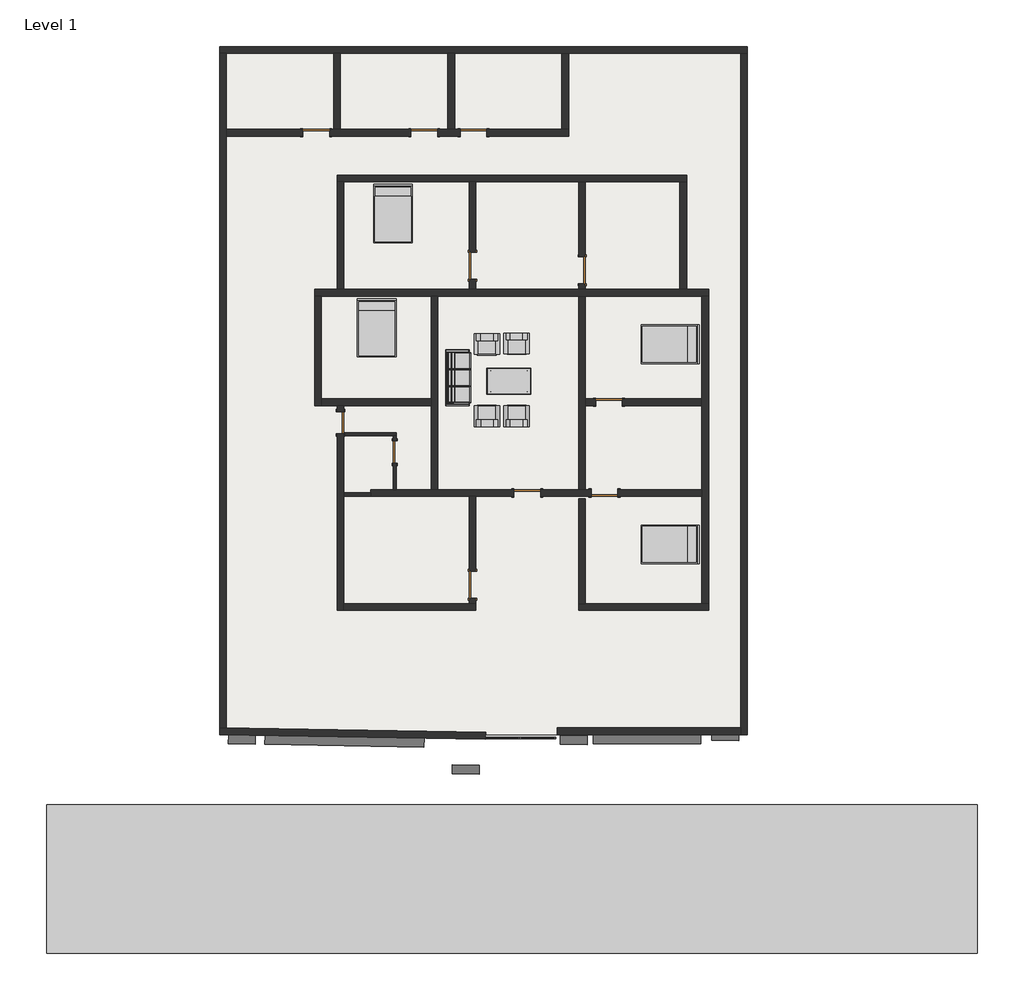
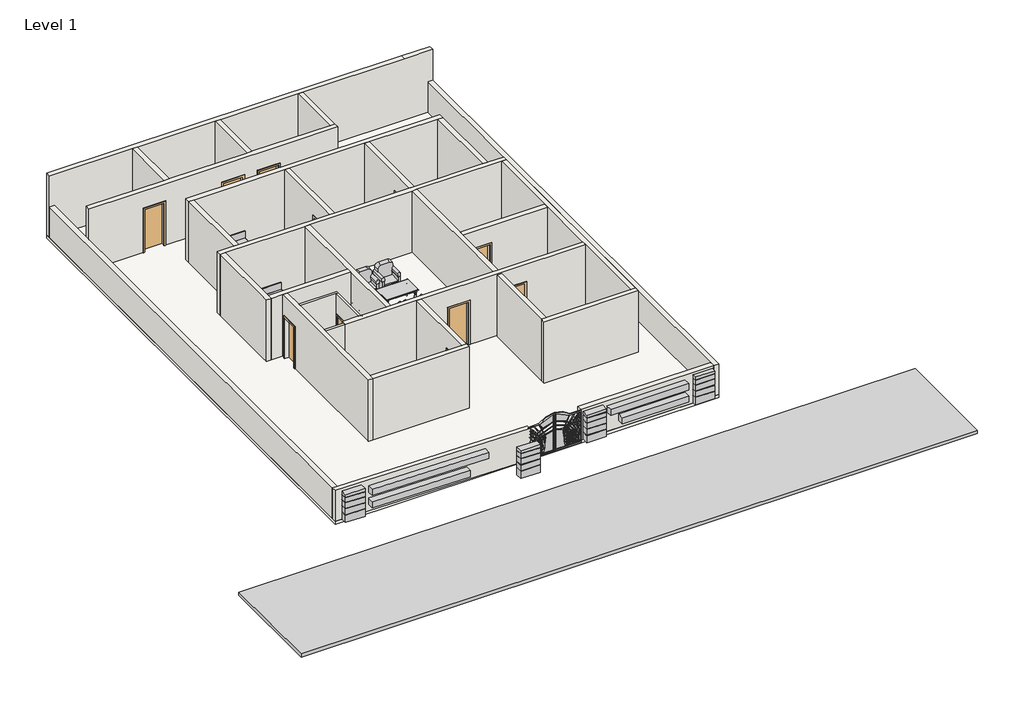
# One storey, incomplete: 30 walls, 11 doors, 10 furniture elements, 8 proxies, 1 slab.
"""IFC4 building model written with IfcOpenShell, lengths in millimetres."""

from ifc_helpers import new_model, si_unit, frame, origin, origin_with_axes, place, context, project, spatial, polyline, outline, extrude, faceted_brep, transform, mapped, element, save
from components import generic_models_6bc30956, generic_models_1_generic_models_1_9302cbdc, generic_models_2_generic_models_2_68b0420d, generic_models_3_generic_models_1_5bebd585, generic_models_4_generic_models_1_1a32cfe3, generic_models_5_generic_models_1_3fb950e5, generic_models_6_generic_models_6_20551735, generic_models_7_generic_models_7_4119f6ec, door_a1484949, door_d8f5dbb5, door_0ca8825f, door_a90ba1ad, furniture_2fc85b74, furniture_29a9adb8, furniture_57072a26, bed_17739_bed_17739_15c61121, chair_lounge_11461_couch_0866092f, dining_table_14755_dining_table_14755_d89cb775

model = new_model("IFC4")

# Units and contexts
model_context = context("Model", 3, world=origin())
ifc_project = project(units=[si_unit("LENGTHUNIT", "METRE", prefix="MILLI")], contexts=[model_context])

# Site, building, storey
site = spatial("IfcSite", under=ifc_project)
building = spatial("IfcBuilding", under=site)
storey = spatial("IfcBuildingStorey", under=building, Name="Level 1", Elevation=0.0)

# Proxies
placement = place(None, origin())
generic_models_shape = generic_models_6bc30956(model_context)
element("IfcBuildingElementProxy", 1, Name="Generic Models", at=placement, inside=storey, context=model_context, shape_type="MappedRepresentation", body=[
    mapped(generic_models_shape, transform((-28.292132, -11258.8237368, 0.0), x_axis=(1.0, 0.0, 0.0), y_axis=(0.0, 1.0, 0.0), z_axis=(0.0, 0.0, 1.0))),
])
generic_models_1_generic_models_1_shape = generic_models_1_generic_models_1_9302cbdc(model_context)
element("IfcBuildingElementProxy", 2, Name="Generic Models 1 : Generic Models 1", ObjectType="Generic Models 1 : Generic Models 1", at=placement, inside=storey, context=model_context, shape_type="MappedRepresentation", body=[
    mapped(generic_models_1_generic_models_1_shape, transform((0.0, 0.0, 0.0), x_axis=(1.0, 0.0, 0.0), y_axis=(0.0, 1.0, 0.0), z_axis=(0.0, 0.0, 1.0))),
])
generic_models_2_generic_models_2_shape = generic_models_2_generic_models_2_68b0420d(model_context)
element("IfcBuildingElementProxy", 3, Name="Generic Models 2 : Generic Models 2", ObjectType="Generic Models 2 : Generic Models 2", at=placement, inside=storey, context=model_context, shape_type="MappedRepresentation", body=[
    mapped(generic_models_2_generic_models_2_shape, transform((0.0, 0.0, 0.0), x_axis=(1.0, 0.0, 0.0), y_axis=(0.0, 1.0, 0.0), z_axis=(0.0, 0.0, 1.0))),
])
generic_models_3_generic_models_1_shape = generic_models_3_generic_models_1_5bebd585(model_context)
element("IfcBuildingElementProxy", 4, Name="Generic Models 3 : Generic Models 1", ObjectType="Generic Models 3 : Generic Models 1", at=placement, inside=storey, context=model_context, shape_type="MappedRepresentation", body=[
    mapped(generic_models_3_generic_models_1_shape, transform((0.0, 0.0, 0.0), x_axis=(1.0, 0.0, 0.0), y_axis=(0.0, 1.0, 0.0), z_axis=(0.0, 0.0, 1.0))),
])
generic_models_4_generic_models_1_shape = generic_models_4_generic_models_1_1a32cfe3(model_context)
element("IfcBuildingElementProxy", 5, Name="Generic Models 4 : Generic Models 1", ObjectType="Generic Models 4 : Generic Models 1", at=placement, inside=storey, context=model_context, shape_type="MappedRepresentation", body=[
    mapped(generic_models_4_generic_models_1_shape, transform((0.0, 0.0, 0.0), x_axis=(1.0, 0.0, 0.0), y_axis=(0.0, 1.0, 0.0), z_axis=(0.0, 0.0, 1.0))),
])
generic_models_5_generic_models_1_shape = generic_models_5_generic_models_1_3fb950e5(model_context)
element("IfcBuildingElementProxy", 6, Name="Generic Models 5 : Generic Models 1", ObjectType="Generic Models 5 : Generic Models 1", at=placement, inside=storey, context=model_context, shape_type="MappedRepresentation", body=[
    mapped(generic_models_5_generic_models_1_shape, transform((0.0, 0.0, 0.0), x_axis=(1.0, 0.0, 0.0), y_axis=(0.0, 1.0, 0.0), z_axis=(0.0, 0.0, 1.0))),
])
generic_models_6_generic_models_6_shape = generic_models_6_generic_models_6_20551735(model_context)
element("IfcBuildingElementProxy", 7, Name="Generic Models 6 : Generic Models 6", ObjectType="Generic Models 6 : Generic Models 6", at=placement, inside=storey, context=model_context, shape_type="MappedRepresentation", body=[
    mapped(generic_models_6_generic_models_6_shape, transform((0.0, 0.0, 0.0), x_axis=(1.0, 0.0, 0.0), y_axis=(0.0, 1.0, 0.0), z_axis=(0.0, 0.0, 1.0))),
])
generic_models_7_generic_models_7_shape = generic_models_7_generic_models_7_4119f6ec(model_context)
element("IfcBuildingElementProxy", 8, Name="Generic Models 7 : Generic Models 7", ObjectType="Generic Models 7 : Generic Models 7", at=placement, inside=storey, context=model_context, shape_type="MappedRepresentation", body=[
    mapped(generic_models_7_generic_models_7_shape, transform((0.0, 0.0, 0.0), x_axis=(1.0, 0.0, 0.0), y_axis=(0.0, 1.0, 0.0), z_axis=(0.0, 0.0, 1.0))),
])

# Doors
door_shape = door_a1484949(model_context)
element("IfcDoor", 9, ObjectType="Single-Flush : 30\" x 80\"", at=placement, inside=storey, context=model_context, shape_type="MappedRepresentation", body=[
    mapped(door_shape, transform((-6124.8057305, -546.3292186, 0.0), x_axis=(0.0, -1.0, 0.0), y_axis=(1.0, 0.0, 0.0), z_axis=(0.0, 0.0, 1.0))),
])
door_2_shape = door_d8f5dbb5(model_context)
element("IfcDoor", 10, ObjectType="Single-Flush : 30\" x 80\"", at=placement, inside=storey, context=model_context, shape_type="MappedRepresentation", body=[
    mapped(door_2_shape, transform((-4276.442132, -1546.4542186, 0.0), x_axis=(0.0, 1.0, 0.0), y_axis=(-1.0, 0.0, 0.0), z_axis=(0.0, 0.0, 1.0))),
])
door_3_shape = door_0ca8825f(model_context)
element("IfcDoor", 11, ObjectType="Single-Flush : 36\" x 84\"", at=placement, inside=storey, context=model_context, shape_type="MappedRepresentation", body=[
    mapped(door_3_shape, transform((-6952.8959326, 9329.2722985, 0.0), x_axis=(1.0, 0.0, 0.0), y_axis=(0.0, 1.0, 0.0), z_axis=(0.0, 0.0, 1.0))),
])
element("IfcDoor", 12, ObjectType="Single-Flush : 36\" x 84\"", at=placement, inside=storey, context=model_context, shape_type="MappedRepresentation", body=[
    mapped(door_3_shape, transform((-3267.5476203, 9329.2722985, 0.0), x_axis=(1.0, 0.0, 0.0), y_axis=(0.0, 1.0, 0.0), z_axis=(0.0, 0.0, 1.0))),
])
element("IfcDoor", 13, ObjectType="Single-Flush : 36\" x 84\"", at=placement, inside=storey, context=model_context, shape_type="MappedRepresentation", body=[
    mapped(door_3_shape, transform((2105.307868, 4644.7957814, 0.0), x_axis=(0.0, -1.0, 0.0), y_axis=(1.0, 0.0, 0.0), z_axis=(0.0, 0.0, 1.0))),
])
element("IfcDoor", 14, ObjectType="Single-Flush : 36\" x 84\"", at=placement, inside=storey, context=model_context, shape_type="MappedRepresentation", body=[
    mapped(door_3_shape, transform((2867.307868, -2937.1042186, 0.0), x_axis=(-1.0, 0.0, 0.0), y_axis=(0.0, -1.0, 0.0), z_axis=(0.0, 0.0, 1.0))),
])
element("IfcDoor", 15, ObjectType="Single-Flush : 36\" x 84\"", at=placement, inside=storey, context=model_context, shape_type="MappedRepresentation", body=[
    mapped(door_3_shape, transform((238.407868, -2937.1042186, 0.0), x_axis=(1.0, 0.0, 0.0), y_axis=(0.0, 1.0, 0.0), z_axis=(0.0, 0.0, 1.0))),
])
door_4_shape = door_a90ba1ad(model_context)
element("IfcDoor", 16, ObjectType="Single-Flush : 36\" x 84\"", at=placement, inside=storey, context=model_context, shape_type="MappedRepresentation", body=[
    mapped(door_4_shape, transform((-1591.1476203, 9329.2722985, 0.0), x_axis=(-1.0, 0.0, 0.0), y_axis=(0.0, -1.0, 0.0), z_axis=(0.0, 0.0, 1.0))),
])
element("IfcDoor", 17, ObjectType="Single-Flush : 36\" x 84\"", at=placement, inside=storey, context=model_context, shape_type="MappedRepresentation", body=[
    mapped(door_4_shape, transform((-1628.492132, 4797.1957814, 0.0), x_axis=(0.0, -1.0, 0.0), y_axis=(1.0, 0.0, 0.0), z_axis=(0.0, 0.0, 1.0))),
])
element("IfcDoor", 18, ObjectType="Single-Flush : 36\" x 84\"", at=placement, inside=storey, context=model_context, shape_type="MappedRepresentation", body=[
    mapped(door_4_shape, transform((3019.707868, 148.9957814, 0.0), x_axis=(-1.0, 0.0, 0.0), y_axis=(0.0, -1.0, 0.0), z_axis=(0.0, 0.0, 1.0))),
])
element("IfcDoor", 19, ObjectType="Single-Flush : 36\" x 84\"", at=placement, inside=storey, context=model_context, shape_type="MappedRepresentation", body=[
    mapped(door_4_shape, transform((-1628.492132, -6061.3042186, 0.0), x_axis=(0.0, -1.0, 0.0), y_axis=(1.0, 0.0, 0.0), z_axis=(0.0, 0.0, 1.0))),
])

# Furniture
furniture_shape = furniture_2fc85b74(model_context)
furniture_2_shape = furniture_29a9adb8(model_context)
furniture_3_shape = furniture_57072a26(model_context)
element("IfcFurniture", 20, at=placement, inside=storey, context=model_context, shape_type="MappedRepresentation", body=[
    mapped(furniture_shape, transform((-1742.792132, 987.1957814, 0.0), x_axis=(0.0, 1.0, 0.0), y_axis=(-1.0, 0.0, 0.0), z_axis=(0.0, 0.0, 1.0))),
    mapped(furniture_2_shape, transform((-1742.792132, 987.1957814, 0.0), x_axis=(0.0, 1.0, 0.0), y_axis=(-1.0, 0.0, 0.0), z_axis=(0.0, 0.0, 1.0))),
    mapped(furniture_3_shape, transform((-1742.792132, 987.1957814, 0.0), x_axis=(0.0, 1.0, 0.0), y_axis=(-1.0, 0.0, 0.0), z_axis=(0.0, 0.0, 1.0))),
])
bed_17739_bed_17739_shape = bed_17739_bed_17739_15c61121(model_context)
element("IfcFurniture", 21, ObjectType="Bed_17739 : Bed_17739", at=placement, inside=storey, context=model_context, shape_type="MappedRepresentation", body=[
    mapped(bed_17739_bed_17739_shape, transform((-4333.592132, 6549.7957814, 0.0), x_axis=(1.0, 0.0, 0.0), y_axis=(0.0, 1.0, 0.0), z_axis=(0.0, 0.0, 1.0))),
])
element("IfcFurniture", 22, ObjectType="Bed_17739 : Bed_17739", at=placement, inside=storey, context=model_context, shape_type="MappedRepresentation", body=[
    mapped(bed_17739_bed_17739_shape, transform((5077.107868, 2130.1957814, 0.0), x_axis=(0.0, -1.0, 0.0), y_axis=(1.0, 0.0, 0.0), z_axis=(0.0, 0.0, 1.0))),
])
element("IfcFurniture", 23, ObjectType="Bed_17739 : Bed_17739", at=placement, inside=storey, context=model_context, shape_type="MappedRepresentation", body=[
    mapped(bed_17739_bed_17739_shape, transform((5077.107868, -4689.7042186, 0.0), x_axis=(0.0, -1.0, 0.0), y_axis=(1.0, 0.0, 0.0), z_axis=(0.0, 0.0, 1.0))),
])
element("IfcFurniture", 24, ObjectType="Bed_17739 : Bed_17739", at=placement, inside=storey, context=model_context, shape_type="MappedRepresentation", body=[
    mapped(bed_17739_bed_17739_shape, transform((-4886.042132, 2663.5957814, 0.0), x_axis=(1.0, 0.0, 0.0), y_axis=(0.0, 1.0, 0.0), z_axis=(0.0, 0.0, 1.0))),
])
chair_lounge_11461_couch_shape = chair_lounge_11461_couch_0866092f(model_context)
element("IfcFurniture", 25, ObjectType="Chair-Lounge_11461 : Couch", at=placement, inside=storey, context=model_context, shape_type="MappedRepresentation", body=[
    mapped(chair_lounge_11461_couch_shape, transform((-1135.6501746, 2478.1239494, 0.0), x_axis=(1.0, 0.0, 0.0), y_axis=(0.0, 1.0, 0.0), z_axis=(0.0, 0.0, 1.0))),
])
element("IfcFurniture", 26, ObjectType="Chair-Lounge_11461 : Couch", at=placement, inside=storey, context=model_context, shape_type="MappedRepresentation", body=[
    mapped(chair_lounge_11461_couch_shape, transform((-1135.6501746, -676.3685812, 0.0), x_axis=(-1.0, 0.0, 0.0), y_axis=(0.0, -1.0, 0.0), z_axis=(0.0, 0.0, 1.0))),
])
element("IfcFurniture", 27, ObjectType="Chair-Lounge_11461 : Couch", at=placement, inside=storey, context=model_context, shape_type="MappedRepresentation", body=[
    mapped(chair_lounge_11461_couch_shape, transform((-125.9107827, -676.3685812, 0.0), x_axis=(-1.0, 0.0, 0.0), y_axis=(0.0, -1.0, 0.0), z_axis=(0.0, 0.0, 1.0))),
])
element("IfcFurniture", 28, ObjectType="Chair-Lounge_11461 : Couch", at=placement, inside=storey, context=model_context, shape_type="MappedRepresentation", body=[
    mapped(chair_lounge_11461_couch_shape, transform((-125.9107827, 2504.7969663, 0.0), x_axis=(1.0, 0.0, 0.0), y_axis=(0.0, 1.0, 0.0), z_axis=(0.0, 0.0, 1.0))),
])
dining_table_14755_dining_table_14755_shape = dining_table_14755_dining_table_14755_d89cb775(model_context)
element("IfcFurniture", 29, ObjectType="Dining_table_14755 : Dining_table_14755", at=placement, inside=storey, context=model_context, shape_type="MappedRepresentation", body=[
    mapped(dining_table_14755_dining_table_14755_shape, transform((-1135.6501746, 415.6957814, 0.0), x_axis=(1.0, 0.0, 0.0), y_axis=(0.0, 1.0, 0.0), z_axis=(0.0, 0.0, 1.0))),
])

# Slab
element("IfcSlab", 30, ObjectType="Generic - 12\"", at=placement, inside=storey, context=model_context, shape_type="SweptSolid", body=[
    extrude(outline(polyline([(7729.3646036, 12262.9722985), (7729.3646036, -11166.6749898), (-10239.8476203, -11166.6749898), (-10239.8476203, 12262.9722985), (7729.3646036, 12262.9722985)])), frame((0.0, 0.0, -152.4), z_axis=(0.0, 0.0, 1.0), x_axis=(1.0, 0.0, 0.0)), (0.0, 0.0, 1.0), 152.4),
])

# Walls
element("IfcWall", 31, ObjectType="4.5\"WALL", at=placement, inside=storey, context=model_context, shape_type="Brep", body=[
    faceted_brep([(-6010.5057305, -994.0042186, 0.0), (-4333.592132, -994.0042186, 0.0), (-4219.292132, -994.0042186, 0.0), (-4219.292132, -994.0042186, 3048.0), (-4333.592132, -994.0042186, 3048.0), (-6010.5057305, -994.0042186, 3048.0), (-6010.5057305, -879.7042186, 0.0), (-6010.5057305, -879.7042186, 3048.0), (-4219.292132, -879.7042186, 3048.0), (-4219.292132, -879.7042186, 0.0)], [[[0, 1, 2, 3, 4, 5]], [[6, 7, 8, 9]], [[2, 1, 0, 6, 9]], [[0, 5, 7, 6]], [[3, 2, 9, 8]], [[5, 4, 3, 8, 7]]]),
])
element("IfcWall", 32, ObjectType="4.5\"WALL", at=placement, inside=storey, context=model_context, shape_type="SweptSolid", body=[
    extrude(outline(polyline([(-994.0042186, 0.0), (-1165.4542186, 0.0), (-1165.4542186, 2032.0), (-1927.4542186, 2032.0), (-1927.4542186, 0.0), (-2822.8042186, 0.0), (-2822.8042186, 3048.0), (-994.0042186, 3048.0), (-994.0042186, 0.0)])), frame((-4333.592132, 0.0, 0.0), z_axis=(1.0, 0.0, 0.0), x_axis=(0.0, 1.0, 0.0)), (0.0, 0.0, 1.0), 114.3),
])
element("IfcWall", 33, ObjectType="4.5\"WALL", at=placement, inside=storey, context=model_context, shape_type="SweptSolid", body=[
    extrude(outline(polyline([(-5096.0236102, -3051.4042186), (-6010.5057305, -3051.4042186), (-6010.5057305, -2937.1042186), (-5096.0236102, -2937.1042186), (-5096.0236102, -3051.4042186)])), origin_with_axes(), (0.0, 0.0, 1.0), 3048.0),
])
element("IfcWall", 34, ObjectType="WALL9\"", at=placement, inside=storey, context=model_context, shape_type="Brep", body=[
    faceted_brep([(-10239.8476203, 12034.3722985, 0.0), (-10011.2476203, 12034.3722985, 0.0), (-6353.6476203, 12034.3722985, 0.0), (-6125.0476203, 12034.3722985, 0.0), (-2467.4476203, 12034.3722985, 0.0), (-2238.8476203, 12034.3722985, 0.0), (1418.7523797, 12034.3722985, 0.0), (1647.3523797, 12034.3722985, 0.0), (7500.7646036, 12034.3722985, 0.0), (7729.3646036, 12034.3722985, 0.0), (7729.3646036, 12034.3722985, 1524.0), (7729.3646036, 12034.3722985, 3048.0), (6410.607868, 12034.3722985, 3048.0), (1647.3523797, 12034.3722985, 3048.0), (1418.7523797, 12034.3722985, 3048.0), (-2238.8476203, 12034.3722985, 3048.0), (-2467.4476203, 12034.3722985, 3048.0), (-6125.0476203, 12034.3722985, 3048.0), (-6353.6476203, 12034.3722985, 3048.0), (-10239.8476203, 12034.3722985, 3048.0), (-10239.8476203, 12034.3722985, 1524.0), (-10239.8476203, 12262.9722985, 0.0), (-10239.8476203, 12262.9722985, 3048.0), (6410.607868, 12262.9722985, 3048.0), (7729.3646036, 12262.9722985, 3048.0), (7729.3646036, 12262.9722985, 0.0)], [[[0, 1, 2, 3, 4, 5, 6, 7, 8, 9, 10, 11, 12, 13, 14, 15, 16, 17, 18, 19, 20]], [[21, 22, 23, 24, 25]], [[9, 8, 7, 6, 5, 4, 3, 2, 1, 0, 21, 25]], [[11, 10, 9, 25, 24]], [[12, 11, 24, 23]], [[19, 18, 17, 16, 15, 14, 13, 12, 23, 22]], [[0, 20, 19, 22, 21]]]),
])
element("IfcWall", 35, ObjectType="WALL9\"", at=placement, inside=storey, context=model_context, shape_type="Brep", body=[
    faceted_brep([(7500.7646036, 12034.3722985, 0.0), (7500.7646036, -10938.0749898, 0.0), (7500.7646036, -11166.6749898, 0.0), (7500.7646036, -11166.6749898, 1524.0), (7500.7646036, -10938.0749898, 1524.0), (7500.7646036, 12034.3722985, 1524.0), (7729.3646036, 12034.3722985, 0.0), (7729.3646036, 12034.3722985, 1524.0), (7729.3646036, -11166.6749898, 1524.0), (7729.3646036, -11166.6749898, 0.0)], [[[0, 1, 2, 3, 4, 5]], [[6, 7, 8, 9]], [[2, 1, 0, 6, 9]], [[5, 4, 3, 8, 7]], [[0, 5, 7, 6]], [[3, 2, 9, 8]]]),
])
element("IfcWall", 36, ObjectType="WALL9\"", at=placement, inside=storey, context=model_context, shape_type="SweptSolid", body=[
    extrude(outline(polyline([(1265.0646036, -10938.0749898), (7500.7646036, -10938.0749898), (7500.7646036, -11166.6749898), (1265.0646036, -11166.6749898), (1265.0646036, -10938.0749898)])), origin_with_axes(), (0.0, 0.0, 1.0), 1524.0),
])
element("IfcWall", 37, ObjectType="WALL9\"", at=placement, inside=storey, context=model_context, shape_type="Brep", body=[
    faceted_brep([(-2810.3476203, 9214.9722985, 0.0), (-2048.3476203, 9214.9722985, 0.0), (-2048.3476203, 9214.9722985, 2133.6), (-1133.9476203, 9214.9722985, 2133.6), (-1133.9476203, 9214.9722985, 0.0), (1647.3523797, 9214.9722985, 0.0), (1647.3523797, 9214.9722985, 3048.0), (-6238.592132, 9214.9722985, 3048.0), (-10011.2476203, 9214.9722985, 3048.0), (-10011.2476203, 9214.9722985, 0.0), (-7410.0959326, 9214.9722985, 0.0), (-7410.0959326, 9214.9722985, 2133.6), (-6495.6959326, 9214.9722985, 2133.6), (-6495.6959326, 9214.9722985, 0.0), (-3724.7476203, 9214.9722985, 0.0), (-3724.7476203, 9214.9722985, 2133.6), (-2810.3476203, 9214.9722985, 2133.6), (-2048.3476203, 9443.5722985, 2133.6), (-2048.3476203, 9443.5722985, 0.0), (-2238.8476203, 9443.5722985, 0.0), (-2467.4476203, 9443.5722985, 0.0), (-2810.3476203, 9443.5722985, 0.0), (-2810.3476203, 9443.5722985, 2133.6), (-3724.7476203, 9443.5722985, 2133.6), (-3724.7476203, 9443.5722985, 0.0), (-6125.0476203, 9443.5722985, 0.0), (-6353.6476203, 9443.5722985, 0.0), (-6495.6959326, 9443.5722985, 0.0), (-6495.6959326, 9443.5722985, 2133.6), (-7410.0959326, 9443.5722985, 2133.6), (-7410.0959326, 9443.5722985, 0.0), (-10011.2476203, 9443.5722985, 0.0), (-10011.2476203, 9443.5722985, 3048.0), (-6353.6476203, 9443.5722985, 3048.0), (-6125.0476203, 9443.5722985, 3048.0), (-2467.4476203, 9443.5722985, 3048.0), (-2238.8476203, 9443.5722985, 3048.0), (1418.7523797, 9443.5722985, 3048.0), (1647.3523797, 9443.5722985, 3048.0), (1647.3523797, 9443.5722985, 0.0), (1418.7523797, 9443.5722985, 0.0), (-1133.9476203, 9443.5722985, 0.0), (-1133.9476203, 9443.5722985, 2133.6)], [[[0, 1, 2, 3, 4, 5, 6, 7, 8, 9, 10, 11, 12, 13, 14, 15, 16]], [[17, 18, 19, 20, 21, 22, 23, 24, 25, 26, 27, 28, 29, 30, 31, 32, 33, 34, 35, 36, 37, 38, 39, 40, 41, 42]], [[10, 9, 31, 30]], [[14, 13, 27, 26, 25, 24]], [[41, 40, 39, 5, 4]], [[21, 20, 19, 18, 1, 0]], [[6, 5, 39, 38]], [[28, 27, 13, 12]], [[29, 28, 12, 11]], [[30, 29, 11, 10]], [[22, 21, 0, 16]], [[23, 22, 16, 15]], [[24, 23, 15, 14]], [[2, 1, 18, 17]], [[3, 2, 17, 42]], [[4, 3, 42, 41]], [[8, 7, 6, 38, 37, 36, 35, 34, 33, 32]], [[9, 8, 32, 31]]]),
])
element("IfcWall", 38, ObjectType="WALL9\"", at=placement, inside=storey, context=model_context, shape_type="SweptSolid", body=[
    extrude(outline(polyline([(1647.3523797, 12034.3722985), (1647.3523797, 9443.5722985), (1418.7523797, 9443.5722985), (1418.7523797, 12034.3722985), (1647.3523797, 12034.3722985)])), origin_with_axes(), (0.0, 0.0, 1.0), 3048.0),
])
element("IfcWall", 39, ObjectType="WALL9\"", at=placement, inside=storey, context=model_context, shape_type="SweptSolid", body=[
    extrude(outline(polyline([(-2467.4476203, 9443.5722985), (-2467.4476203, 12034.3722985), (-2238.8476203, 12034.3722985), (-2238.8476203, 9443.5722985), (-2467.4476203, 9443.5722985)])), origin_with_axes(), (0.0, 0.0, 1.0), 3048.0),
])
element("IfcWall", 40, ObjectType="WALL9\"", at=placement, inside=storey, context=model_context, shape_type="SweptSolid", body=[
    extrude(outline(polyline([(-6353.6476203, 9443.5722985), (-6353.6476203, 12034.3722985), (-6125.0476203, 12034.3722985), (-6125.0476203, 9443.5722985), (-6353.6476203, 9443.5722985)])), origin_with_axes(), (0.0, 0.0, 1.0), 3048.0),
])
element("IfcWall", 41, ObjectType="WALL9\"", at=placement, inside=storey, context=model_context, shape_type="Brep", body=[
    faceted_brep([(-6238.592132, 7654.6957814, 0.0), (-6009.992132, 7654.6957814, 0.0), (-1742.792132, 7654.6957814, 0.0), (-1514.192132, 7654.6957814, 0.0), (1991.007868, 7654.6957814, 0.0), (2219.607868, 7654.6957814, 0.0), (5432.707868, 7654.6957814, 0.0), (5661.307868, 7654.6957814, 0.0), (5661.307868, 7654.6957814, 3048.0), (5432.707868, 7654.6957814, 3048.0), (2219.607868, 7654.6957814, 3048.0), (1991.007868, 7654.6957814, 3048.0), (-1514.192132, 7654.6957814, 3048.0), (-1742.792132, 7654.6957814, 3048.0), (-6009.992132, 7654.6957814, 3048.0), (-6238.592132, 7654.6957814, 3048.0), (-6238.592132, 7883.2957814, 0.0), (-6238.592132, 7883.2957814, 3048.0), (5661.307868, 7883.2957814, 3048.0), (5661.307868, 7883.2957814, 0.0)], [[[0, 1, 2, 3, 4, 5, 6, 7, 8, 9, 10, 11, 12, 13, 14, 15]], [[16, 17, 18, 19]], [[7, 6, 5, 4, 3, 2, 1, 0, 16, 19]], [[0, 15, 17, 16]], [[15, 14, 13, 12, 11, 10, 9, 8, 18, 17]], [[8, 7, 19, 18]]]),
])
element("IfcWall", 42, ObjectType="WALL9\"", at=placement, inside=storey, context=model_context, shape_type="SweptSolid", body=[
    extrude(outline(polyline([(-6238.592132, 3997.0957814), (-6238.592132, 7654.6957814), (-6009.992132, 7654.6957814), (-6009.992132, 3997.0957814), (-6238.592132, 3997.0957814)])), origin_with_axes(), (0.0, 0.0, 1.0), 3048.0),
])
element("IfcWall", 43, ObjectType="WALL9\"", at=placement, inside=storey, context=model_context, shape_type="SweptSolid", body=[
    extrude(outline(polyline([(4339.9957814, 2133.6), (4339.9957814, 0.0), (3997.0957814, 0.0), (3997.0957814, 3048.0), (7654.6957814, 3048.0), (7654.6957814, 0.0), (5254.3957814, 0.0), (5254.3957814, 2133.6), (4339.9957814, 2133.6)])), frame((-1742.792132, 0.0, 0.0), z_axis=(1.0, 0.0, 0.0), x_axis=(0.0, 1.0, 0.0)), (0.0, 0.0, 1.0), 228.6),
])
element("IfcWall", 44, ObjectType="WALL9\"", at=placement, inside=storey, context=model_context, shape_type="SweptSolid", body=[
    extrude(outline(polyline([(4187.5957814, 2133.6), (4187.5957814, 0.0), (3997.0957814, 0.0), (3997.0957814, 3048.0), (7654.6957814, 3048.0), (7654.6957814, 0.0), (5101.9957814, 0.0), (5101.9957814, 2133.6), (4187.5957814, 2133.6)])), frame((1991.007868, 0.0, 0.0), z_axis=(1.0, 0.0, 0.0), x_axis=(0.0, 1.0, 0.0)), (0.0, 0.0, 1.0), 228.6),
])
element("IfcWall", 45, ObjectType="WALL9\"", at=placement, inside=storey, context=model_context, shape_type="Brep", body=[
    faceted_brep([(-7000.592132, 3768.4957814, 0.0), (-6771.992132, 3768.4957814, 0.0), (-3038.192132, 3768.4957814, 0.0), (-2809.592132, 3768.4957814, 0.0), (1991.007868, 3768.4957814, 0.0), (2219.607868, 3768.4957814, 0.0), (6182.007868, 3768.4957814, 0.0), (6410.607868, 3768.4957814, 0.0), (6410.607868, 3768.4957814, 3048.0), (6182.007868, 3768.4957814, 3048.0), (2219.607868, 3768.4957814, 3048.0), (1991.007868, 3768.4957814, 3048.0), (-2809.592132, 3768.4957814, 3048.0), (-3038.192132, 3768.4957814, 3048.0), (-6771.992132, 3768.4957814, 3048.0), (-7000.592132, 3768.4957814, 3048.0), (-7000.592132, 3997.0957814, 0.0), (-7000.592132, 3997.0957814, 3048.0), (-6238.592132, 3997.0957814, 3048.0), (-6009.992132, 3997.0957814, 3048.0), (-1742.792132, 3997.0957814, 3048.0), (-1514.192132, 3997.0957814, 3048.0), (1991.007868, 3997.0957814, 3048.0), (2219.607868, 3997.0957814, 3048.0), (5432.707868, 3997.0957814, 3048.0), (5661.307868, 3997.0957814, 3048.0), (6410.607868, 3997.0957814, 3048.0), (6410.607868, 3997.0957814, 0.0), (5661.307868, 3997.0957814, 0.0), (5432.707868, 3997.0957814, 0.0), (2219.607868, 3997.0957814, 0.0), (1991.007868, 3997.0957814, 0.0), (-1514.192132, 3997.0957814, 0.0), (-1742.792132, 3997.0957814, 0.0), (-6009.992132, 3997.0957814, 0.0), (-6238.592132, 3997.0957814, 0.0)], [[[0, 1, 2, 3, 4, 5, 6, 7, 8, 9, 10, 11, 12, 13, 14, 15]], [[16, 17, 18, 19, 20, 21, 22, 23, 24, 25, 26, 27, 28, 29, 30, 31, 32, 33, 34, 35]], [[7, 6, 5, 4, 3, 2, 1, 0, 16, 35, 34, 33, 32, 31, 30, 29, 28, 27]], [[0, 15, 17, 16]], [[15, 14, 13, 12, 11, 10, 9, 8, 26, 25, 24, 23, 22, 21, 20, 19, 18, 17]], [[8, 7, 27, 26]]]),
])
element("IfcWall", 46, ObjectType="WALL9\"", at=placement, inside=storey, context=model_context, shape_type="SweptSolid", body=[
    extrude(outline(polyline([(0.0, 2219.607868), (0.0, 2562.507868), (2133.6, 2562.507868), (2133.6, 3476.907868), (0.0, 3476.907868), (0.0, 6182.007868), (3048.0, 6182.007868), (3048.0, 2219.607868), (0.0, 2219.607868)])), frame((0.0, 34.6957814, 0.0), z_axis=(0.0, 1.0, 0.0), x_axis=(0.0, 0.0, 1.0)), (0.0, 0.0, 1.0), 228.6),
])
element("IfcWall", 47, ObjectType="WALL9\"", at=placement, inside=storey, context=model_context, shape_type="Brep", body=[
    faceted_brep([(-7000.592132, 3768.4957814, 0.0), (-7000.592132, 34.6957814, 0.0), (-7000.592132, 34.6957814, 3048.0), (-7000.592132, 3768.4957814, 3048.0), (-6771.992132, 3768.4957814, 0.0), (-6771.992132, 3768.4957814, 3048.0), (-6771.992132, 263.2957814, 3048.0), (-6771.992132, 34.6957814, 3048.0), (-6771.992132, 34.6957814, 0.0), (-6771.992132, 263.2957814, 0.0)], [[[0, 1, 2, 3]], [[4, 5, 6, 7, 8, 9]], [[1, 0, 4, 9, 8]], [[0, 3, 5, 4]], [[2, 1, 8, 7]], [[3, 2, 7, 6, 5]]]),
])
element("IfcWall", 48, ObjectType="WALL9\"", at=placement, inside=storey, context=model_context, shape_type="Brep", body=[
    faceted_brep([(-6771.992132, 34.6957814, 0.0), (-6239.1057305, 34.6957814, 0.0), (-6010.5057305, 34.6957814, 0.0), (-3038.192132, 34.6957814, 0.0), (-3038.192132, 34.6957814, 3048.0), (-6010.5057305, 34.6957814, 3048.0), (-6239.1057305, 34.6957814, 3048.0), (-6771.992132, 34.6957814, 3048.0), (-6771.992132, 263.2957814, 0.0), (-6771.992132, 263.2957814, 3048.0), (-3038.192132, 263.2957814, 3048.0), (-3038.192132, 263.2957814, 0.0)], [[[0, 1, 2, 3, 4, 5, 6, 7]], [[8, 9, 10, 11]], [[3, 2, 1, 0, 8, 11]], [[0, 7, 9, 8]], [[4, 3, 11, 10]], [[7, 6, 5, 4, 10, 9]]]),
])
element("IfcWall", 49, ObjectType="WALL9\"", at=placement, inside=storey, context=model_context, shape_type="Brep", body=[
    faceted_brep([(-3038.192132, 3768.4957814, 0.0), (-3038.192132, 263.2957814, 0.0), (-3038.192132, 34.6957814, 0.0), (-3038.192132, -2822.8042186, 0.0), (-3038.192132, -2822.8042186, 3048.0), (-3038.192132, 34.6957814, 3048.0), (-3038.192132, 263.2957814, 3048.0), (-3038.192132, 3768.4957814, 3048.0), (-2809.592132, 3768.4957814, 0.0), (-2809.592132, 3768.4957814, 3048.0), (-2809.592132, -2822.8042186, 3048.0), (-2809.592132, -2822.8042186, 0.0)], [[[0, 1, 2, 3, 4, 5, 6, 7]], [[8, 9, 10, 11]], [[3, 2, 1, 0, 8, 11]], [[0, 7, 9, 8]], [[4, 3, 11, 10]], [[7, 6, 5, 4, 10, 9]]]),
])
element("IfcWall", 50, ObjectType="WALL9\"", at=placement, inside=storey, context=model_context, shape_type="Brep", body=[
    faceted_brep([(1991.007868, 3768.4957814, 0.0), (1991.007868, -2822.8042186, 0.0), (1991.007868, -2822.8042186, 3048.0), (1991.007868, 3768.4957814, 3048.0), (2219.607868, 3768.4957814, 0.0), (2219.607868, 3768.4957814, 3048.0), (2219.607868, 263.2957814, 3048.0), (2219.607868, 34.6957814, 3048.0), (2219.607868, -2822.8042186, 3048.0), (2219.607868, -2822.8042186, 0.0), (2219.607868, 34.6957814, 0.0), (2219.607868, 263.2957814, 0.0)], [[[0, 1, 2, 3]], [[4, 5, 6, 7, 8, 9, 10, 11]], [[1, 0, 4, 11, 10, 9]], [[0, 3, 5, 4]], [[2, 1, 9, 8]], [[3, 2, 8, 7, 6, 5]]]),
])
element("IfcWall", 51, ObjectType="WALL9\"", at=placement, inside=storey, context=model_context, shape_type="Brep", body=[
    faceted_brep([(-6239.1057305, -927.3292186, 2032.0), (-6239.1057305, -927.3292186, 0.0), (-6239.1057305, -6937.6042186, 0.0), (-6239.1057305, -6937.6042186, 3048.0), (-6239.1057305, 34.6957814, 3048.0), (-6239.1057305, 34.6957814, 0.0), (-6239.1057305, -165.3292186, 0.0), (-6239.1057305, -165.3292186, 2032.0), (-6010.5057305, -6937.6042186, 0.0), (-6010.5057305, -6709.0042186, 0.0), (-6010.5057305, -3051.4042186, 0.0), (-6010.5057305, -2937.1042186, 0.0), (-6010.5057305, -994.0042186, 0.0), (-6010.5057305, -927.3292186, 0.0), (-6010.5057305, -927.3292186, 2032.0), (-6010.5057305, -165.3292186, 2032.0), (-6010.5057305, -165.3292186, 0.0), (-6010.5057305, 34.6957814, 0.0), (-6010.5057305, 34.6957814, 3048.0), (-6010.5057305, -879.7042186, 3048.0), (-6010.5057305, -994.0042186, 3048.0), (-6010.5057305, -2937.1042186, 3048.0), (-6010.5057305, -3051.4042186, 3048.0), (-6010.5057305, -6709.0042186, 3048.0), (-6010.5057305, -6937.6042186, 3048.0)], [[[0, 1, 2, 3, 4, 5, 6, 7]], [[8, 9, 10, 11, 12, 13, 14, 15, 16, 17, 18, 19, 20, 21, 22, 23, 24]], [[6, 5, 17, 16]], [[2, 1, 13, 12, 11, 10, 9, 8]], [[5, 4, 18, 17]], [[3, 2, 8, 24]], [[14, 13, 1, 0]], [[15, 14, 0, 7]], [[16, 15, 7, 6]], [[4, 3, 24, 23, 22, 21, 20, 19, 18]]]),
])
element("IfcWall", 52, ObjectType="WALL9\"", at=placement, inside=storey, context=model_context, shape_type="Brep", body=[
    faceted_brep([(-1514.192132, -6709.0042186, 0.0), (-1742.792132, -6709.0042186, 0.0), (-6010.5057305, -6709.0042186, 0.0), (-6010.5057305, -6709.0042186, 3048.0), (-1742.792132, -6709.0042186, 3048.0), (-1514.192132, -6709.0042186, 3048.0), (-1514.192132, -6937.6042186, 0.0), (-1514.192132, -6937.6042186, 3048.0), (-6010.5057305, -6937.6042186, 3048.0), (-6010.5057305, -6937.6042186, 0.0)], [[[0, 1, 2, 3, 4, 5]], [[6, 7, 8, 9]], [[2, 1, 0, 6, 9]], [[3, 2, 9, 8]], [[0, 5, 7, 6]], [[5, 4, 3, 8, 7]]]),
])
element("IfcWall", 53, ObjectType="WALL9\"", at=placement, inside=storey, context=model_context, shape_type="Brep", body=[
    faceted_brep([(695.607868, -3051.4042186, 2133.6), (695.607868, -3051.4042186, 0.0), (2410.107868, -3051.4042186, 0.0), (2410.107868, -3051.4042186, 2133.6), (3324.507868, -3051.4042186, 2133.6), (3324.507868, -3051.4042186, 0.0), (6182.007868, -3051.4042186, 0.0), (6182.007868, -3051.4042186, 3048.0), (-1514.192132, -3051.4042186, 3048.0), (-1742.792132, -3051.4042186, 3048.0), (-5096.0236102, -3051.4042186, 3048.0), (-5096.0236102, -3051.4042186, 0.0), (-1742.792132, -3051.4042186, 0.0), (-1514.192132, -3051.4042186, 0.0), (-218.792132, -3051.4042186, 0.0), (-218.792132, -3051.4042186, 2133.6), (2410.107868, -2822.8042186, 0.0), (2219.607868, -2822.8042186, 0.0), (1991.007868, -2822.8042186, 0.0), (695.607868, -2822.8042186, 0.0), (695.607868, -2822.8042186, 2133.6), (-218.792132, -2822.8042186, 2133.6), (-218.792132, -2822.8042186, 0.0), (-2809.592132, -2822.8042186, 0.0), (-3038.192132, -2822.8042186, 0.0), (-4219.292132, -2822.8042186, 0.0), (-4333.592132, -2822.8042186, 0.0), (-5096.0236102, -2822.8042186, 0.0), (-5096.0236102, -2822.8042186, 3048.0), (-4333.592132, -2822.8042186, 3048.0), (-4219.292132, -2822.8042186, 3048.0), (-3038.192132, -2822.8042186, 3048.0), (-2809.592132, -2822.8042186, 3048.0), (1991.007868, -2822.8042186, 3048.0), (2219.607868, -2822.8042186, 3048.0), (6182.007868, -2822.8042186, 3048.0), (6182.007868, -2822.8042186, 0.0), (3324.507868, -2822.8042186, 0.0), (3324.507868, -2822.8042186, 2133.6), (2410.107868, -2822.8042186, 2133.6), (-5096.0236102, -2937.1042186, 0.0), (-5096.0236102, -2937.1042186, 3048.0)], [[[0, 1, 2, 3, 4, 5, 6, 7, 8, 9, 10, 11, 12, 13, 14, 15]], [[16, 17, 18, 19, 20, 21, 22, 23, 24, 25, 26, 27, 28, 29, 30, 31, 32, 33, 34, 35, 36, 37, 38, 39]], [[37, 36, 6, 5]], [[2, 1, 19, 18, 17, 16]], [[14, 13, 12, 11, 40, 27, 26, 25, 24, 23, 22]], [[11, 10, 41, 28, 27, 40]], [[3, 2, 16, 39]], [[4, 3, 39, 38]], [[5, 4, 38, 37]], [[20, 19, 1, 0]], [[21, 20, 0, 15]], [[22, 21, 15, 14]], [[10, 9, 8, 7, 35, 34, 33, 32, 31, 30, 29, 28, 41]], [[7, 6, 36, 35]]]),
])
element("IfcWall", 54, ObjectType="WALL9\"", at=placement, inside=storey, context=model_context, shape_type="Brep", body=[
    faceted_brep([(6410.607868, -6709.0042186, 0.0), (6182.007868, -6709.0042186, 0.0), (2219.607868, -6709.0042186, 0.0), (1991.007868, -6709.0042186, 0.0), (1991.007868, -6709.0042186, 3048.0), (2219.607868, -6709.0042186, 3048.0), (6182.007868, -6709.0042186, 3048.0), (6410.607868, -6709.0042186, 3048.0), (6410.607868, -6937.6042186, 0.0), (6410.607868, -6937.6042186, 3048.0), (1991.007868, -6937.6042186, 3048.0), (1991.007868, -6937.6042186, 0.0)], [[[0, 1, 2, 3, 4, 5, 6, 7]], [[8, 9, 10, 11]], [[3, 2, 1, 0, 8, 11]], [[4, 3, 11, 10]], [[7, 6, 5, 4, 10, 9]], [[0, 7, 9, 8]]]),
])
element("IfcWall", 55, ObjectType="WALL9\"", at=placement, inside=storey, context=model_context, shape_type="SweptSolid", body=[
    extrude(outline(polyline([(2219.607868, -3127.6042186), (2219.607868, -6709.0042186), (1991.007868, -6709.0042186), (1991.007868, -3127.6042186), (2219.607868, -3127.6042186)])), origin_with_axes(), (0.0, 0.0, 1.0), 3048.0),
])
element("IfcWall", 56, ObjectType="WALL9\"", at=placement, inside=storey, context=model_context, shape_type="SweptSolid", body=[
    extrude(outline(polyline([(-6518.5042186, 2133.6), (-6518.5042186, 0.0), (-6709.0042186, 0.0), (-6709.0042186, 3048.0), (-3051.4042186, 3048.0), (-3051.4042186, 0.0), (-5604.1042186, 0.0), (-5604.1042186, 2133.6), (-6518.5042186, 2133.6)])), frame((-1742.792132, 0.0, 0.0), z_axis=(1.0, 0.0, 0.0), x_axis=(0.0, 1.0, 0.0)), (0.0, 0.0, 1.0), 228.6),
])
element("IfcWall", 57, ObjectType="WALL9\"", at=placement, inside=storey, context=model_context, shape_type="Brep", body=[
    faceted_brep([(-1182.1197274, -11094.1482821, 0.0), (-10011.2476203, -10940.0352815, 0.0), (-10239.8476203, -10936.0450537, 0.0), (-10239.8476203, -10936.0450537, 1524.0), (-10011.2476203, -10940.0352815, 1524.0), (-1182.1197274, -11094.1482821, 1524.0), (-1186.1093475, -11322.7134653, 0.0), (-1186.1093475, -11322.7134653, 1524.0), (-10239.8476203, -11164.6798759, 1524.0), (-10239.8476203, -11164.6798759, 0.0)], [[[0, 1, 2, 3, 4, 5]], [[6, 7, 8, 9]], [[2, 1, 0, 6, 9]], [[5, 4, 3, 8, 7]], [[0, 5, 7, 6]], [[3, 2, 9, 8]]]),
])
element("IfcWall", 58, ObjectType="WALL9\"", at=placement, inside=storey, context=model_context, shape_type="SweptSolid", body=[
    extrude(outline(polyline([(5432.707868, 3997.0957814), (5432.707868, 7654.6957814), (5661.307868, 7654.6957814), (5661.307868, 3997.0957814), (5432.707868, 3997.0957814)])), origin_with_axes(), (0.0, 0.0, 1.0), 3048.0),
])
element("IfcWall", 59, ObjectType="WALL9\"", at=placement, inside=storey, context=model_context, shape_type="Brep", body=[
    faceted_brep([(6182.007868, 3768.4957814, 0.0), (6182.007868, 263.2957814, 0.0), (6182.007868, 34.6957814, 0.0), (6182.007868, -2822.8042186, 0.0), (6182.007868, -3051.4042186, 0.0), (6182.007868, -6709.0042186, 0.0), (6182.007868, -6709.0042186, 3048.0), (6182.007868, -3051.4042186, 3048.0), (6182.007868, -2822.8042186, 3048.0), (6182.007868, 34.6957814, 3048.0), (6182.007868, 263.2957814, 3048.0), (6182.007868, 3768.4957814, 3048.0), (6410.607868, 3768.4957814, 0.0), (6410.607868, 3768.4957814, 3048.0), (6410.607868, -6709.0042186, 3048.0), (6410.607868, -6709.0042186, 0.0)], [[[0, 1, 2, 3, 4, 5, 6, 7, 8, 9, 10, 11]], [[12, 13, 14, 15]], [[5, 4, 3, 2, 1, 0, 12, 15]], [[11, 10, 9, 8, 7, 6, 14, 13]], [[0, 11, 13, 12]], [[6, 5, 15, 14]]]),
])
element("IfcWall", 60, ObjectType="WALL9\"", at=placement, inside=storey, context=model_context, shape_type="Brep", body=[
    faceted_brep([(-10239.8476203, 12034.3722985, 0.0), (-10239.8476203, -10936.0450537, 0.0), (-10239.8476203, -10936.0450537, 1524.0), (-10239.8476203, 12034.3722985, 1524.0), (-10011.2476203, 12034.3722985, 0.0), (-10011.2476203, 12034.3722985, 1524.0), (-10011.2476203, -10940.0352815, 1524.0), (-10011.2476203, -10940.0352815, 0.0), (-10011.2476203, 9214.9722985, 0.0), (-10011.2476203, 9443.5722985, 0.0)], [[[0, 1, 2, 3]], [[4, 5, 6, 7, 8, 9]], [[1, 0, 4, 9, 8, 7]], [[3, 2, 6, 5]], [[0, 3, 5, 4]], [[2, 1, 7, 6]]]),
])

save(model, "model.ifc")

# Revit data of these elements
# Type
#   m.s. sheet = none
#   2" x2" pipe = none
#   1"x1"pipe = none
#   Default Elevation = 0
# Type "Single-Flush : 30\" x 80\""
#   Type Mark = "5"
#   Construction Type Id = "MDOOR"
#   Assembly Code = "C1020"
#   Analytic Construction = "Metal"
#   Thickness = 0' - 2"
#   Heat Transfer Coefficient (U) = 0.651978 BTU/(h·ft²·°F)
#   Height = 6' - 8"
#   Trim Projection Ext = 0' - 1"
#   Trim Projection Int = 0' - 1"
#   Trim Width = 0' - 3"
#   Width = 2' - 6"
#   Define Thermal Properties by = 1
#   Define Thermal Properties by = 1
#   Door Material = Door - Panel
#   Frame Material = Door - Frame
#   Visual Light Transmittance = 0
#   Solar Heat Gain Coefficient = 0
#   Function = (empty or 0)
#   Wall Closure = (empty or 0)
# Type "Single-Flush : 36\" x 84\""
#   Type Mark = "1"
#   Construction Type Id = "MDOOR"
#   Assembly Code = "C1020"
#   Analytic Construction = "Metal"
#   Thickness = 0' - 2"
#   Heat Transfer Coefficient (U) = 0.651978 BTU/(h·ft²·°F)
#   Height = 7' - 0"
#   Trim Projection Ext = 0' - 1"
#   Trim Projection Int = 0' - 1"
#   Trim Width = 0' - 3"
#   Width = 3' - 0"
#   Define Thermal Properties by = 1
#   Define Thermal Properties by = 1
#   Door Material = Door - Panel
#   Frame Material = Door - Frame
#   Visual Light Transmittance = 0
#   Solar Heat Gain Coefficient = 0
#   Function = (empty or 0)
#   Wall Closure = (empty or 0)
# Type
#   Width [instance] = 6' - 3.19685"
#   Default Elevation = 0
# Type "Bed_17739 : Bed_17739"
#   Default Elevation = 0
# Type "Chair-Lounge_11461 : Couch"
#   Default Elevation = 0
#   Assembly Code = ""
# Type "Dining_table_14755 : Dining_table_14755"
#   Lengte [instance default] = 4' - 11.05512"
#   Breedte [instance default] = 2' - 11.43307"
#   Tafelblad = none
#   Poten = none
#   Default Elevation = 0
# Type "Generic - 12\""
#   Assembly Code = "B1010"
#   Function = 0
#   Layers, outside or top first: 0' - 6" no material (function 1)
# Type "4.5\"WALL"
#   Assembly Code = "B2010"
#   Layers, outside or top first: 0' - 4 1/2" no material (function 1)
# Type "WALL9\""
#   Assembly Code = "B2010"
#   Layers, outside or top first: 0' - 9" no material (function 1)
# Element 1 (IfcBuildingElementProxy)
#   Phase Created = New Construction
#   Materials on its faces: "r1"
# Element 2 (IfcBuildingElementProxy, "Generic Models 1 : Generic Models 1")
#   Phase Created = New Construction
#   Materials on its faces: "Parking Stripe"
# Element 3 (IfcBuildingElementProxy, "Generic Models 2 : Generic Models 2")
#   Phase Created = New Construction
#   Materials on its faces: "Blanket"
# Element 4 (IfcBuildingElementProxy, "Generic Models 3 : Generic Models 1")
#   Phase Created = New Construction
#   Materials on its faces: "Parking Stripe"
# Element 5 (IfcBuildingElementProxy, "Generic Models 4 : Generic Models 1")
#   Phase Created = New Construction
#   Materials on its faces: "Parking Stripe"
# Element 6 (IfcBuildingElementProxy, "Generic Models 5 : Generic Models 1")
#   Phase Created = New Construction
#   Materials on its faces: "Parking Stripe"
# Element 7 (IfcBuildingElementProxy, "Generic Models 6 : Generic Models 6")
#   Phase Created = New Construction
#   Materials on its faces: "Blanket"
# Element 8 (IfcBuildingElementProxy, "Generic Models 7 : Generic Models 7")
#   Phase Created = New Construction
# Elements 9, 10 (IfcDoor, "Single-Flush : 30\" x 80\"")
#   Phase Created = New Construction
#   Materials on its faces: "Door - Frame", "Door - Panel"
# Elements 11, 12, 13, 14, 15, 16, 17, 18, 19 (IfcDoor, "Single-Flush : 36\" x 84\"")
#   Phase Created = New Construction
#   Materials on its faces: "Door - Frame", "Door - Panel"
# Element 20 (IfcFurniture)
#   Width = 6' - 3.19685"
#   Phase Created = New Construction
# Elements 21, 22, 23, 24 (IfcFurniture, "Bed_17739 : Bed_17739")
#   Phase Created = New Construction
#   Materials on its faces: "legs", "sheets", "bed frame", "Blanket"
# Elements 25, 26, 27, 28 (IfcFurniture, "Chair-Lounge_11461 : Couch")
#   Phase Created = New Construction
# Element 29 (IfcFurniture, "Dining_table_14755 : Dining_table_14755")
#   Lengte = 4' - 11.05512"
#   Breedte = 2' - 11.43307"
#   Phase Created = New Construction
# Element 30 (IfcSlab, "Generic - 12\"")
#   Height Offset From Level = 0' - 0"
#   Phase Created = New Construction
#   Materials on its faces: "Default Floor"
# Elements 31, 32, 33 (IfcWall, "4.5\"WALL")
#   Top Offset = 0' - 0"
#   Base Offset = 0' - 0"
#   Unconnected Height = 10' - 0"
#   wall height = 10' - 0"
#   Phase Created = New Construction
#   Base Constraint = Level 1
#   Materials on its faces: "Default Wall"
# Element 34 (IfcWall, "WALL9\"")
#   Top Offset = 0' - 0"
#   Base Offset = 0' - 0"
#   Unconnected Height = 10' - 0"
#   wall height = 10' - 0"
#   Phase Created = New Construction
#   Base Constraint = Level 1
#   Materials on its faces: "Default Wall", "Wood - Stained", "WALL7"
# Elements 35, 36, 57, 60 (IfcWall, "WALL9\"")
#   Top Offset = 0' - 0"
#   Base Offset = 0' - 0"
#   Unconnected Height = 5' - 0"
#   wall height = 5' - 0"
#   Phase Created = New Construction
#   Base Constraint = Level 1
#   Materials on its faces: "Default Wall", "Wood - Stained"
# Elements 37, 38, 40, 41, 42, 45, 47, 51, 52, 53, 54, 58, 59 (IfcWall, "WALL9\"")
#   Top Offset = 0' - 0"
#   Base Offset = 0' - 0"
#   Unconnected Height = 10' - 0"
#   wall height = 10' - 0"
#   Phase Created = New Construction
#   Base Constraint = Level 1
#   Materials on its faces: "Default Wall", "WALL7"
# Elements 39, 43, 44, 46, 48, 49, 50, 55, 56 (IfcWall, "WALL9\"")
#   Top Offset = 0' - 0"
#   Base Offset = 0' - 0"
#   Unconnected Height = 10' - 0"
#   wall height = 10' - 0"
#   Phase Created = New Construction
#   Base Constraint = Level 1
#   Materials on its faces: "Default Wall"
# Materials
#   "Door - Panel": class "Wood", colour RGB 210 159 95, transparency 0, Cost = 0
#   "Door - Frame": colour RGB 118 70 51, transparency 0, Cost = 0
#   "r1": class "Generic", colour RGB 120 120 120, transparency 0, Cost = 0
#   "Parking Stripe": class "Paint", colour RGB 250 250 91, transparency 0, Cost = 0
#   "Blanket": class "System", colour RGB 59 0 1, transparency 0, Cost = 0
#   "legs": colour RGB 90 73 37, transparency 0, Cost = 0
#   "sheets": colour RGB 200 195 176, transparency 0, Cost = 0
#   "bed frame": colour RGB 90 73 37, transparency 0, Cost = 0
#   "Default Floor": colour RGB 128 128 128, transparency 0, Cost = 0
#   "Default Wall": colour RGB 128 128 128, transparency 0, Cost = 0
#   "Wood - Stained": class "Wood", colour RGB 224 178 126, transparency 0, Cost = 0
#   "WALL7": class "Generic", colour RGB 200 200 200, transparency 0, Cost = 0
